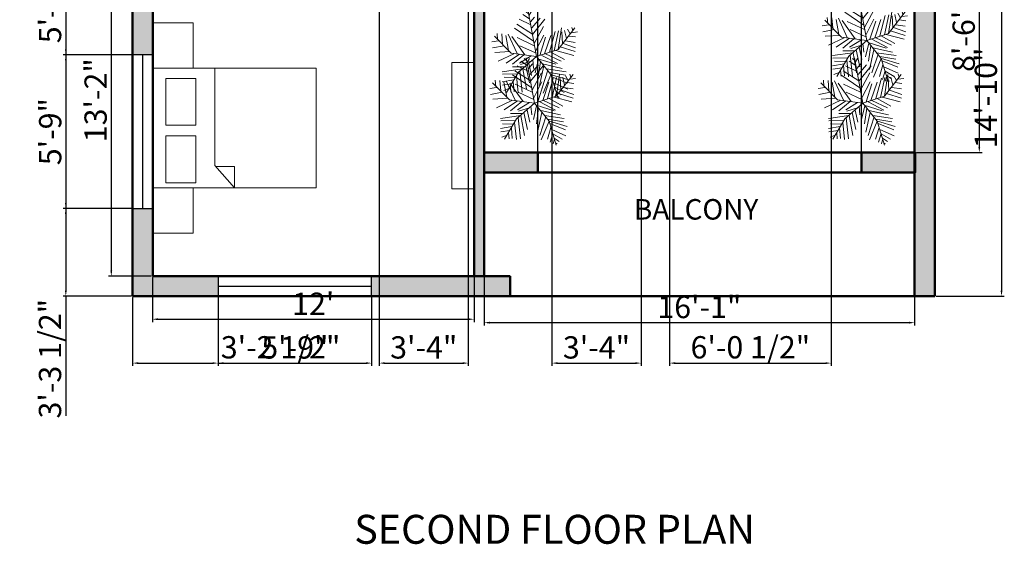
# Model space of a CAD drawing. Units: inches. Extents: x 1344 to 2521, y 3236 to 4924.
# Tile 4 of 14: x 1968 to 2410, y 3236 to 3472. Entities that reach past the tile are written whole.
import ezdxf

# ---------------------------------------------------------------- set-up
doc = ezdxf.new("R2010")
doc.units = ezdxf.units.IN
for name, color, linetype, lineweight in [('A-ANNO-DIMS', 2, 'Continuous', 18), ('A-ANNO-TEXT', 7, 'Continuous', 25), ('A-AREA-IDEN', 3, 'Continuous', 18), ('A-FURN', 130, 'Continuous', 18), ('A-GLAZ', 150, 'Continuous', 25), ('A-WALL', 31, 'Continuous', 50), ('A-WALL-PATT', 8, 'Continuous', 13), ('L-PLNT', 82, 'Continuous', 13)]:
    doc.layers.add(name, color=color, linetype=linetype, lineweight=lineweight)
doc.styles.get("Standard").update_dxf_attribs({"font": 'arial.ttf'})
doc.dimstyles.new('ISO-25', dxfattribs={"dimtxt": 10, "dimasz": 2.5, "dimexe": 1.25, "dimexo": 0.625, "dimtad": 1, "dimdec": 0, "dimlunit": 4, "dimtxsty": 'Standard', "dimcen": 2.5, "dimadec": 0, "dimazin": 0, "dimtfac": 1, "dimtdec": 0, "dimtmove": 0, "dimatfit": 3, "dimfxl": 1, "dimarcsym": 0})

# ---------------------------------------------------------------- blocks, each defined once
blk = doc.blocks.new('*U8')
for p, q in [((-8.737, 47.138), (-17.069, 52.711)), ((-10.186, 53.64), (-13.084, 55.962)), ((0, 0), (-10.5, 57)), ((-9.099, 51.782), (-6.563, 55.962)), ((-7.65, 43.423), (-2.578, 49.46)), ((-5.114, 28.097), (-24.676, 40.636)), ((-7.288, 39.707), (-21.778, 46.673)), ((-5.839, 35.992), (4.667, 48.067)), ((-5.114, 27.632), (10.463, 46.673)), ((-2.941, 16.486), (8.652, 37.85)), ((-31.5, 4.5), (-52.5, 25.5)), ((-48.585, 21.131), (-49.309, 29.026)), ((-43.513, 28.561), (-42.427, 15.558)), ((-38.442, 26.239), (-34.819, 7.663)), ((-35.544, 28.097), (-24.314, 3.947)), ((-14.533, 2.09), (-30.834, 25.31)), ((-3.665, 19.273), (-27.574, 35.527)), ((-1.129, 6.734), (9.014, 26.704)), ((10.101, 3.483), (17.708, 26.239)), ((16.259, 5.805), (23.142, 31.348)), ((22.055, 7.198), (27.489, 32.277)), ((27, 9), (48, 36)), ((27.127, 9.056), (31.112, 35.992)), ((31.836, 30.883), (32.561, 16.486)), ((35.096, 32.741), (37.27, 22.524)), ((38.719, 34.134), (41.979, 28.561)), ((40.53, 25.775), (48.862, 24.846)), ((43.791, 29.954), (51.036, 30.883)), ((44.153, 36.456), (45.239, 32.741)), ((-47.498, 19.737), (-55.83, 18.344)), ((-40.615, 13.7), (-55.105, 10.913)), ((-24.314, 23.917), (-2.941, 13.7)), ((-20.691, 13.7), (-1.129, 4.876)), ((3.942, 1.625), (11.187, 24.381)), ((29.662, 12.307), (48.137, 6.269)), ((33.285, 16.486), (48.862, 10.913)), ((36.183, 19.737), (48.137, 17.88)), ((-33.37, 6.269), (-52.207, 5.34)), ((-28.299, 3.483), (-47.86, -5.805)), ((-21.416, 3.018), (-38.079, -8.128)), ((0, 0), (-31.5, 4.5)), ((-15.982, 2.09), (-30.11, -9.521)), ((0, 0), (-22.5, -19.5)), ((-6.563, 1.161), (-21.416, -8.128)), ((0, 0), (27, 9)), ((0, 0), (18, -22.5)), ((6.478, 1.625), (26.04, -8.592)), ((11.187, 3.483), (30.749, -5.805)), ((18.07, 5.805), (35.096, -3.483)), ((24.229, 7.663), (46.688, 1.625)), ((-6.563, -5.805), (-19.967, -9.985)), ((-13.446, -11.378), (-8.737, -32.741)), ((-9.461, -8.592), (-6.201, -23.453)), ((-4.752, -3.483), (-3.665, -14.629)), ((2.493, -3.019), (-1.491, -20.202)), ((1.769, -2.555), (24.229, -9.521)), ((5.029, -6.27), (2.131, -25.775)), ((9.014, -11.378), (3.58, -35.992)), ((7.565, -9.056), (32.198, -14.629)), ((-17.431, -15.094), (-42.789, -18.809)), ((-24.314, -21.596), (-42.427, -22.06)), ((-22.5, -19.5), (-37.5, -45)), ((-15.257, -12.772), (-30.11, -12.772)), ((-25.038, -23.918), (-22.865, -45.281)), ((-20.691, -18.345), (-17.793, -44.352)), ((-17.069, -15.094), (-12.721, -40.172)), ((14.085, -16.951), (6.478, -40.172)), ((18.07, -22.524), (8.289, -45.745)), ((12.274, -15.094), (36.907, -18.809)), ((16.259, -19.738), (36.183, -22.989)), ((18, -22.5), (27, -52.5)), ((18.433, -22.524), (40.53, -29.026)), ((-28.299, -29.026), (-42.789, -31.348)), ((-30.834, -34.135), (-42.427, -35.528)), ((-26.849, -26.24), (-40.253, -25.775)), ((-29.023, -30.884), (-27.936, -43.887)), ((20.244, -30.419), (15.897, -44.816)), ((19.157, -25.311), (38.719, -33.206)), ((21.331, -32.741), (39.081, -40.636)), ((-34.457, -39.708), (-40.978, -42.494)), ((-32.646, -36.921), (-31.921, -44.352)), ((22.78, -37.85), (19.519, -48.532)), ((22.78, -38.314), (34.372, -44.816)), ((24.591, -45.745), (23.142, -50.854)), ((24.591, -43.423), (30.749, -47.603)), ((26.764, -49.925), (28.213, -50.854))]:
    blk.add_line(p, q)
blk = doc.blocks.new('*D54')
at = {"layer": 'A-ANNO-DIMS', "color": 0, "lineweight": -2, "transparency": 16777216}
for p, q in [((2026.74, 3514.45), (2007.52, 3514.45)), ((2008.77, 3511.95), (2008.77, 3358.97)), ((2026.74, 3356.47), (2007.52, 3356.47))]:
    blk.add_line(p, q, dxfattribs=at)
at = {"layer": 'A-ANNO-DIMS', "color": 0, "lineweight": 100, "transparency": 16777216}
for points in [[(2008.35, 3511.95), (2009.18, 3511.95), (2008.77, 3514.45)], [(2008.35, 3358.97), (2009.18, 3358.97), (2008.77, 3356.47)]]:
    blk.add_solid(points, dxfattribs=at)
at = {"layer": 'Defpoints', "color": 0, "lineweight": 100, "transparency": 16777216}
for p in [(2027.36, 3514.45), (2008.77, 3356.47), (2027.36, 3356.47)]:
    blk.add_point(p, dxfattribs=at)
at = {"layer": 'A-ANNO-DIMS', "color": 0, "transparency": 16777216, "insert": (2003.03, 3435.46), "char_height": 10, "attachment_point": 5, "rotation": 90}
blk.add_mtext('13\'-2"', dxfattribs=at)
blk = doc.blocks.new('*D55')
at = {"layer": 'A-ANNO-DIMS', "color": 0, "lineweight": -2, "transparency": 16777216}
for p, q in [((2027.24, 3355.85), (2027.24, 3335.92)), ((2171.6, 3355.85), (2171.6, 3335.92)), ((2029.74, 3337.17), (2169.1, 3337.17))]:
    blk.add_line(p, q, dxfattribs=at)
at = {"layer": 'A-ANNO-DIMS', "color": 0, "lineweight": 100, "transparency": 16777216}
for points in [[(2029.74, 3337.59), (2029.74, 3336.75), (2027.24, 3337.17)], [(2169.1, 3337.59), (2169.1, 3336.75), (2171.6, 3337.17)]]:
    blk.add_solid(points, dxfattribs=at)
at = {"layer": 'Defpoints', "color": 0, "lineweight": 100, "transparency": 16777216}
for p in [(2027.24, 3356.47), (2171.6, 3356.47), (2171.6, 3337.17)]:
    blk.add_point(p, dxfattribs=at)
at = {"layer": 'A-ANNO-DIMS', "color": 0, "transparency": 16777216, "insert": (2099.42, 3342.81), "char_height": 10, "attachment_point": 5}
blk.add_mtext("12'", dxfattribs=at)
blk = doc.blocks.new('*D56')
at = {"layer": 'A-ANNO-DIMS', "color": 0, "lineweight": -2, "transparency": 16777216}
for p, q in [((2176.1, 3355.85), (2176.1, 3334.38)), ((2369.36, 3355.89), (2369.36, 3334.38)), ((2178.6, 3335.63), (2366.86, 3335.63))]:
    blk.add_line(p, q, dxfattribs=at)
at = {"layer": 'A-ANNO-DIMS', "color": 0, "lineweight": 100, "transparency": 16777216}
for points in [[(2178.6, 3336.04), (2178.6, 3335.21), (2176.1, 3335.63)], [(2366.86, 3336.04), (2366.86, 3335.21), (2369.36, 3335.63)]]:
    blk.add_solid(points, dxfattribs=at)
at = {"layer": 'Defpoints', "color": 0, "lineweight": 100, "transparency": 16777216}
for p in [(2176.1, 3356.47), (2369.36, 3356.51), (2369.36, 3335.63)]:
    blk.add_point(p, dxfattribs=at)
at = {"layer": 'A-ANNO-DIMS', "color": 0, "transparency": 16777216, "insert": (2272.73, 3341.36), "char_height": 10, "attachment_point": 5}
blk.add_mtext('16\'-1"', dxfattribs=at)
blk = doc.blocks.new('*D59')
at = {"layer": 'A-ANNO-DIMS', "color": 0, "lineweight": -2, "transparency": 16777216}
for p, q in [((2369.99, 3514.45), (2399.65, 3514.45)), ((2398.4, 3511.95), (2398.4, 3414.51)), ((2370.19, 3412.01), (2399.65, 3412.01))]:
    blk.add_line(p, q, dxfattribs=at)
at = {"layer": 'A-ANNO-DIMS', "color": 0, "lineweight": 100, "transparency": 16777216}
for points in [[(2397.98, 3511.95), (2398.82, 3511.95), (2398.4, 3514.45)], [(2397.98, 3414.51), (2398.82, 3414.51), (2398.4, 3412.01)]]:
    blk.add_solid(points, dxfattribs=at)
at = {"layer": 'Defpoints', "color": 0, "lineweight": 100, "transparency": 16777216}
for p in [(2369.36, 3514.45), (2369.57, 3412.01), (2398.4, 3412.01)]:
    blk.add_point(p, dxfattribs=at)
at = {"layer": 'A-ANNO-DIMS', "color": 0, "transparency": 16777216, "insert": (2392.67, 3463.23), "char_height": 10, "attachment_point": 5, "rotation": 90}
blk.add_mtext('8\'-6"', dxfattribs=at)
blk = doc.blocks.new('BED-DOUBLE')
for p, q in [((27.95, 53.78), (27.95, 9.98)), ((27.95, 9.98), (36.68, 0)), ((36.68, 9.56), (28.32, 9.56)), ((36.68, 0), (36.68, 9.56))]:
    blk.add_line(p, q)
for points in [[(0, 0), (73.35, 0), (73.35, 53.78), (0, 53.78)], [(5.91, 28.08), (19.39, 28.08), (19.39, 49.13), (5.91, 49.13)], [(5.91, 2.27), (19.39, 2.27), (19.39, 23.31), (5.91, 23.31)]]:
    blk.add_lwpolyline(points, close=True)
blk = doc.blocks.new('*D186')
at = {"layer": 'A-ANNO-DIMS', "color": 0, "lineweight": -2, "transparency": 16777216}
for p, q in [((2017.74, 3763.43), (1987.11, 3763.43)), ((1988.36, 3760.93), (1988.36, 3350.01)), ((2017.74, 3347.51), (1987.11, 3347.51))]:
    blk.add_line(p, q, dxfattribs=at)
at = {"layer": 'A-ANNO-DIMS', "color": 0, "lineweight": 100, "transparency": 16777216}
for points in [[(1987.95, 3760.93), (1988.78, 3760.93), (1988.36, 3763.43)], [(1987.95, 3350.01), (1988.78, 3350.01), (1988.36, 3347.51)]]:
    blk.add_solid(points, dxfattribs=at)
at = {"layer": 'Defpoints', "color": 0, "lineweight": 100, "transparency": 16777216}
for p in [(2018.36, 3763.43), (1988.36, 3347.51), (2018.36, 3347.51)]:
    blk.add_point(p, dxfattribs=at)
at = {"layer": 'A-ANNO-DIMS', "color": 0, "transparency": 16777216, "insert": (1982.63, 3555.47), "char_height": 10, "attachment_point": 5, "rotation": 90}
blk.add_mtext('34\'-8"', dxfattribs=at)
blk = doc.blocks.new('*D200')
at = {"layer": 'A-ANNO-DIMS', "color": 0, "lineweight": -2, "transparency": 16777216}
for p, q in [((2017.74, 3527.47), (1987.11, 3527.47)), ((1988.36, 3524.97), (1988.36, 3458.32)), ((2017.74, 3455.82), (1987.11, 3455.82))]:
    blk.add_line(p, q, dxfattribs=at)
at = {"layer": 'A-ANNO-DIMS', "color": 0, "lineweight": 100, "transparency": 16777216}
for points in [[(1987.95, 3524.97), (1988.78, 3524.97), (1988.36, 3527.47)], [(1987.95, 3458.32), (1988.78, 3458.32), (1988.36, 3455.82)]]:
    blk.add_solid(points, dxfattribs=at)
at = {"layer": 'Defpoints', "color": 0, "lineweight": 100, "transparency": 16777216}
for p in [(2018.36, 3527.47), (1988.36, 3455.82), (2018.36, 3455.82)]:
    blk.add_point(p, dxfattribs=at)
at = {"layer": 'A-ANNO-DIMS', "color": 0, "transparency": 16777216, "insert": (1982.57, 3491.65), "char_height": 10, "attachment_point": 5, "rotation": 90}
blk.add_mtext('5\'-11 1/2"', dxfattribs=at)
blk = doc.blocks.new('*D201')
at = {"layer": 'A-ANNO-DIMS', "color": 0, "lineweight": -2, "transparency": 16777216}
for p, q in [((2017.74, 3455.82), (1987.11, 3455.82)), ((1988.36, 3453.32), (1988.36, 3389.4)), ((2017.74, 3386.9), (1987.11, 3386.9))]:
    blk.add_line(p, q, dxfattribs=at)
at = {"layer": 'A-ANNO-DIMS', "color": 0, "lineweight": 100, "transparency": 16777216}
for points in [[(1987.95, 3453.32), (1988.78, 3453.32), (1988.36, 3455.82)], [(1987.95, 3389.4), (1988.78, 3389.4), (1988.36, 3386.9)]]:
    blk.add_solid(points, dxfattribs=at)
at = {"layer": 'Defpoints', "color": 0, "lineweight": 100, "transparency": 16777216}
for p in [(2018.36, 3455.82), (1988.36, 3386.9), (2018.36, 3386.9)]:
    blk.add_point(p, dxfattribs=at)
at = {"layer": 'A-ANNO-DIMS', "color": 0, "transparency": 16777216, "insert": (1982.63, 3421.36), "char_height": 10, "attachment_point": 5, "rotation": 90}
blk.add_mtext('5\'-9"', dxfattribs=at)
blk = doc.blocks.new('*D202')
at = {"layer": 'A-ANNO-DIMS', "color": 0, "lineweight": -2, "transparency": 16777216}
for p, q in [((2017.74, 3386.9), (1987.11, 3386.9)), ((1988.36, 3384.4), (1988.36, 3350.01)), ((2017.74, 3347.51), (1987.11, 3347.51)), ((1988.36, 3347.51), (1988.36, 3293.88))]:
    blk.add_line(p, q, dxfattribs=at)
at = {"layer": 'A-ANNO-DIMS', "color": 0, "lineweight": 100, "transparency": 16777216}
for points in [[(1987.95, 3384.4), (1988.78, 3384.4), (1988.36, 3386.9)], [(1987.95, 3350.01), (1988.78, 3350.01), (1988.36, 3347.51)]]:
    blk.add_solid(points, dxfattribs=at)
at = {"layer": 'Defpoints', "color": 0, "lineweight": 100, "transparency": 16777216}
for p in [(2018.36, 3386.9), (1988.36, 3347.51), (2018.36, 3347.51)]:
    blk.add_point(p, dxfattribs=at)
at = {"layer": 'A-ANNO-DIMS', "color": 0, "transparency": 16777216, "insert": (1982.56, 3319.45), "char_height": 10, "attachment_point": 5, "rotation": 90}
blk.add_mtext('3\'-3 1/2"', dxfattribs=at)
blk = doc.blocks.new('*D205')
at = {"layer": 'A-ANNO-DIMS', "color": 0, "lineweight": -2, "transparency": 16777216}
for p, q in [((2378.99, 3525.36), (2409.61, 3525.36)), ((2408.36, 3522.86), (2408.36, 3350.01)), ((2378.99, 3347.51), (2409.61, 3347.51))]:
    blk.add_line(p, q, dxfattribs=at)
at = {"layer": 'A-ANNO-DIMS', "color": 0, "lineweight": 100, "transparency": 16777216}
for points in [[(2407.95, 3522.86), (2408.78, 3522.86), (2408.36, 3525.36)], [(2407.95, 3350.01), (2408.78, 3350.01), (2408.36, 3347.51)]]:
    blk.add_solid(points, dxfattribs=at)
at = {"layer": 'Defpoints', "color": 0, "lineweight": 100, "transparency": 16777216}
for p in [(2378.36, 3525.36), (2378.36, 3347.51), (2408.36, 3347.51)]:
    blk.add_point(p, dxfattribs=at)
at = {"layer": 'A-ANNO-DIMS', "color": 0, "transparency": 16777216, "insert": (2402.63, 3436.44), "char_height": 10, "attachment_point": 5, "rotation": 90}
blk.add_mtext('14\'-10"', dxfattribs=at)
blk = doc.blocks.new('*D206')
at = {"layer": 'A-ANNO-DIMS', "color": 0, "lineweight": -2, "transparency": 16777216}
for p, q in [((2018.36, 3346.89), (2018.36, 3316.22)), ((2056.7, 3346.85), (2056.7, 3316.22)), ((2020.86, 3317.47), (2054.2, 3317.47)), ((2056.7, 3317.47), (2110.32, 3317.47))]:
    blk.add_line(p, q, dxfattribs=at)
at = {"layer": 'A-ANNO-DIMS', "color": 0, "lineweight": 100, "transparency": 16777216}
for points in [[(2020.86, 3317.89), (2020.86, 3317.06), (2018.36, 3317.47)], [(2054.2, 3317.89), (2054.2, 3317.06), (2056.7, 3317.47)]]:
    blk.add_solid(points, dxfattribs=at)
at = {"layer": 'Defpoints', "color": 0, "lineweight": 100, "transparency": 16777216}
for p in [(2018.36, 3347.51), (2056.7, 3347.47), (2056.7, 3317.47)]:
    blk.add_point(p, dxfattribs=at)
at = {"layer": 'A-ANNO-DIMS', "color": 0, "transparency": 16777216, "insert": (2084.76, 3323.27), "char_height": 10, "attachment_point": 5}
blk.add_mtext('3\'-2 1/2"', dxfattribs=at)
blk = doc.blocks.new('*D207')
at = {"layer": 'A-ANNO-DIMS', "color": 0, "lineweight": -2, "transparency": 16777216}
for p, q in [((2056.7, 3346.85), (2056.7, 3316.22)), ((2125.62, 3346.85), (2125.62, 3316.22)), ((2059.2, 3317.47), (2123.12, 3317.47))]:
    blk.add_line(p, q, dxfattribs=at)
at = {"layer": 'A-ANNO-DIMS', "color": 0, "lineweight": 100, "transparency": 16777216}
for points in [[(2059.2, 3317.89), (2059.2, 3317.06), (2056.7, 3317.47)], [(2123.12, 3317.89), (2123.12, 3317.06), (2125.62, 3317.47)]]:
    blk.add_solid(points, dxfattribs=at)
at = {"layer": 'Defpoints', "color": 0, "lineweight": 100, "transparency": 16777216}
for p in [(2056.7, 3347.47), (2125.62, 3347.47), (2125.62, 3317.47)]:
    blk.add_point(p, dxfattribs=at)
at = {"layer": 'A-ANNO-DIMS', "color": 0, "transparency": 16777216, "insert": (2091.16, 3323.2), "char_height": 10, "attachment_point": 5}
blk.add_mtext('5\'-9"', dxfattribs=at)
blk = doc.blocks.new('*D209')
at = {"layer": 'A-ANNO-DIMS', "color": 0, "lineweight": -2, "transparency": 16777216}
for p, q in [((2129.02, 3619.06), (2129.02, 3316.22)), ((2169.02, 3619.06), (2169.02, 3316.22)), ((2131.52, 3317.47), (2166.52, 3317.47))]:
    blk.add_line(p, q, dxfattribs=at)
at = {"layer": 'A-ANNO-DIMS', "color": 0, "lineweight": 100, "transparency": 16777216}
for points in [[(2131.52, 3317.89), (2131.52, 3317.06), (2129.02, 3317.47)], [(2166.52, 3317.89), (2166.52, 3317.06), (2169.02, 3317.47)]]:
    blk.add_solid(points, dxfattribs=at)
at = {"layer": 'Defpoints', "color": 0, "lineweight": 100, "transparency": 16777216}
for p in [(2129.02, 3619.69), (2169.02, 3619.69), (2169.02, 3317.47)]:
    blk.add_point(p, dxfattribs=at)
at = {"layer": 'A-ANNO-DIMS', "color": 0, "transparency": 16777216, "insert": (2149.02, 3323.21), "char_height": 10, "attachment_point": 5}
blk.add_mtext('3\'-4"', dxfattribs=at)
blk = doc.blocks.new('*D215')
at = {"layer": 'A-ANNO-DIMS', "color": 0, "lineweight": -2, "transparency": 16777216}
for p, q in [((2206.56, 3513.82), (2206.56, 3316.22)), ((2246.56, 3513.82), (2246.56, 3316.22)), ((2209.06, 3317.47), (2244.06, 3317.47))]:
    blk.add_line(p, q, dxfattribs=at)
at = {"layer": 'A-ANNO-DIMS', "color": 0, "lineweight": 100, "transparency": 16777216}
for points in [[(2209.06, 3317.89), (2209.06, 3317.06), (2206.56, 3317.47)], [(2244.06, 3317.89), (2244.06, 3317.06), (2246.56, 3317.47)]]:
    blk.add_solid(points, dxfattribs=at)
at = {"layer": 'Defpoints', "color": 0, "lineweight": 100, "transparency": 16777216}
for p in [(2206.56, 3514.45), (2246.56, 3514.45), (2246.56, 3317.47)]:
    blk.add_point(p, dxfattribs=at)
at = {"layer": 'A-ANNO-DIMS', "color": 0, "transparency": 16777216, "insert": (2226.56, 3323.21), "char_height": 10, "attachment_point": 5}
blk.add_mtext('3\'-4"', dxfattribs=at)
blk = doc.blocks.new('*D216')
at = {"layer": 'A-ANNO-DIMS', "color": 0, "lineweight": -2, "transparency": 16777216}
for p, q in [((2176.1, 3403.64), (2176.1, 3794.68)), ((2178.6, 3793.43), (2197.7, 3793.43)), ((2200.2, 3403.64), (2200.2, 3794.68)), ((2200.2, 3793.43), (2230.7, 3793.43))]:
    blk.add_line(p, q, dxfattribs=at)
at = {"layer": 'A-ANNO-DIMS', "color": 0, "lineweight": 100, "transparency": 16777216}
for points in [[(2178.6, 3793.85), (2178.6, 3793.02), (2176.1, 3793.43)], [(2197.7, 3793.85), (2197.7, 3793.02), (2200.2, 3793.43)]]:
    blk.add_solid(points, dxfattribs=at)
at = {"layer": 'Defpoints', "color": 0, "lineweight": 100, "transparency": 16777216}
for p in [(2200.2, 3793.43), (2176.1, 3403.01), (2200.2, 3403.01)]:
    blk.add_point(p, dxfattribs=at)
at = {"layer": 'A-ANNO-DIMS', "color": 0, "transparency": 16777216, "insert": (2216.7, 3799.16), "char_height": 10, "attachment_point": 5}
blk.add_mtext('2\'-0"', dxfattribs=at)
blk = doc.blocks.new('*D217')
at = {"layer": 'A-ANNO-DIMS', "color": 0, "lineweight": -2, "transparency": 16777216}
for p, q in [((2200.2, 3403.64), (2200.2, 3794.68)), ((2202.7, 3793.43), (2342.96, 3793.43)), ((2345.46, 3403.64), (2345.46, 3794.68))]:
    blk.add_line(p, q, dxfattribs=at)
at = {"layer": 'A-ANNO-DIMS', "color": 0, "lineweight": 100, "transparency": 16777216}
for points in [[(2202.7, 3793.85), (2202.7, 3793.02), (2200.2, 3793.43)], [(2342.96, 3793.85), (2342.96, 3793.02), (2345.46, 3793.43)]]:
    blk.add_solid(points, dxfattribs=at)
at = {"layer": 'Defpoints', "color": 0, "lineweight": 100, "transparency": 16777216}
for p in [(2345.46, 3793.43), (2200.2, 3403.01), (2345.46, 3403.01)]:
    blk.add_point(p, dxfattribs=at)
at = {"layer": 'A-ANNO-DIMS', "color": 0, "transparency": 16777216, "insert": (2272.83, 3799.23), "char_height": 10, "attachment_point": 5}
blk.add_mtext('12\'-1 1/2"', dxfattribs=at)
blk = doc.blocks.new('*D218')
at = {"layer": 'A-ANNO-DIMS', "color": 0, "lineweight": -2, "transparency": 16777216}
for p, q in [((2259.38, 3518.32), (2259.38, 3316.22)), ((2331.86, 3518.32), (2331.86, 3316.22)), ((2261.88, 3317.47), (2329.36, 3317.47))]:
    blk.add_line(p, q, dxfattribs=at)
at = {"layer": 'A-ANNO-DIMS', "color": 0, "lineweight": 100, "transparency": 16777216}
for points in [[(2261.88, 3317.89), (2261.88, 3317.06), (2259.38, 3317.47)], [(2329.36, 3317.89), (2329.36, 3317.06), (2331.86, 3317.47)]]:
    blk.add_solid(points, dxfattribs=at)
at = {"layer": 'Defpoints', "color": 0, "lineweight": 100, "transparency": 16777216}
for p in [(2259.38, 3518.95), (2331.86, 3518.95), (2331.86, 3317.47)]:
    blk.add_point(p, dxfattribs=at)
at = {"layer": 'A-ANNO-DIMS', "color": 0, "transparency": 16777216, "insert": (2295.62, 3323.27), "char_height": 10, "attachment_point": 5}
blk.add_mtext('6\'-0 1/2"', dxfattribs=at)

msp = doc.modelspace()

# ---------------------------------------------------------------- hatches: boundary and pattern name
at = {"layer": 'A-WALL-PATT'}
h = msp.add_hatch(color=256, dxfattribs=at)
h.dxf.hatch_style = 1
h.paths.add_polyline_path([(2193.45, 3763.43), (2126.57, 3763.43), (2126.57, 3754.43), (2193.45, 3754.43)])
h.paths.add_polyline_path([(2057.65, 3763.43), (2018.36, 3763.43), (2018.36, 3608.87), (2027.36, 3608.87), (2027.36, 3754.43), (2057.65, 3754.43)])
h.paths.add_polyline_path([(2266.48, 3763.43), (2226.56, 3763.43), (2226.56, 3754.43), (2266.48, 3754.43)])
h.paths.add_polyline_path([(2378.36, 3763.43), (2335.41, 3763.43), (2335.41, 3754.43), (2369.36, 3754.43), (2369.36, 3594.28), (2378.36, 3594.28)])
h.paths.add_polyline_path([(2369.36, 3610.02), (2250.29, 3610.02), (2250.29, 3605.52), (2369.36, 3605.52)])
h.paths.add_polyline_path([(2250.29, 3610.02), (2245.79, 3610.02), (2245.79, 3605.52), (2250.29, 3605.52)])
h.paths.add_polyline_path([(2250.29, 3754.43), (2245.79, 3754.43), (2245.79, 3655.04), (2250.29, 3655.04)])
h.paths.add_polyline_path([(2176.1, 3754.43), (2171.6, 3754.43), (2171.6, 3624.19), (2171.35, 3624.19), (2169.02, 3624.19), (2169.02, 3619.69), (2176.1, 3619.69)])
h.paths.add_polyline_path([(2129.02, 3624.19), (2122.52, 3624.19), (2122.52, 3619.69), (2129.02, 3619.69)])
h.paths.add_polyline_path([(2091.69, 3624.19), (2027.36, 3624.19), (2027.36, 3619.69), (2091.72, 3619.69, -0.012876), (2091.69, 3620.84)])
h.paths.add_polyline_path([(2250.29, 3615.04), (2245.79, 3615.04), (2245.79, 3610.02), (2250.29, 3610.02)])
h.paths.add_polyline_path([(2027.36, 3580.89), (2018.36, 3580.89), (2018.36, 3555.45), (2027.36, 3555.45)])
h.paths.add_polyline_path([(2027.36, 3527.47), (2018.36, 3527.47), (2018.36, 3455.82), (2027.36, 3455.82)])
h.paths.add_polyline_path([(2093.06, 3517.8, -0.012876), (2093.09, 3518.95), (2027.36, 3518.95), (2027.36, 3514.45), (2093.06, 3514.45)])
h.paths.add_polyline_path([(2118.02, 3573.32), (2110.02, 3573.32), (2110.02, 3573.28), (2080.51, 3573.28), (2027.36, 3573.32), (2027.36, 3568.82), (2118.02, 3568.82)])
h.paths.add_polyline_path([(2122.52, 3624.19), (2114.02, 3624.19), (2114.02, 3620.84), (2114.02, 3619.69), (2118.02, 3619.69), (2118.02, 3518.95), (2122.52, 3518.95)])
h.paths.add_polyline_path([(2129.02, 3518.95), (2115.39, 3518.95), (2115.39, 3517.8), (2115.39, 3514.45), (2129.02, 3514.45)])
h.paths.add_polyline_path([(2027.36, 3386.9), (2018.36, 3386.9), (2018.36, 3347.51), (2056.7, 3347.51), (2056.7, 3356.47), (2027.36, 3356.47)])
h.paths.add_polyline_path([(2187.76, 3356.47), (2168.81, 3356.47), (2149.67, 3356.47), (2125.62, 3356.47), (2125.62, 3347.51), (2176.1, 3347.51), (2187.76, 3347.51)])
h.paths.add_polyline_path([(2378.36, 3525.36), (2369.36, 3525.36), (2369.36, 3497.27), (2369.36, 3412.01), (2369.57, 3412.01), (2369.57, 3403.01), (2369.36, 3356.51), (2369.36, 3347.51), (2378.36, 3347.51)])
h.paths.add_polyline_path([(2369.36, 3412.01), (2345.46, 3412.01), (2345.46, 3403.01), (2369.36, 3403.01)])
h.paths.add_polyline_path([(2206.56, 3518.95), (2176.1, 3518.95), (2176.1, 3514.45), (2206.56, 3514.45)])
h.paths.add_polyline_path([(2130.92, 3560.64), (2239.92, 3560.64), (2239.92, 3579.62), (2130.92, 3579.62)], flags=9)
h.paths.add_polyline_path([(2271.24, 3730.09), (2345.91, 3730.09), (2345.91, 3749.07), (2271.24, 3749.07)], flags=9)
h.paths.add_polyline_path([(2051.28, 3467.76), (2122.39, 3467.76), (2122.39, 3502.26), (2051.28, 3502.26)], flags=9)
h.paths.add_polyline_path([(2033.92, 3520.24), (2083.56, 3520.24), (2083.56, 3539.22), (2033.92, 3539.22)], flags=9)
h.paths.add_polyline_path([(2030.69, 3603.57), (2080.34, 3603.57), (2080.34, 3622.55), (2030.69, 3622.55)], flags=9)
h.paths.add_polyline_path([(2175.78, 3699.42), (2225.43, 3699.42), (2225.43, 3718.41), (2175.78, 3718.41)], flags=9)
h.paths.add_polyline_path([(2051.88, 3718.72), (2122.99, 3718.72), (2122.99, 3753.22), (2051.88, 3753.22)], flags=9)
h = msp.add_hatch(color=256, dxfattribs=at)
h.dxf.hatch_style = 1
h.paths.add_polyline_path([(2200.2, 3412.01), (2176.1, 3412.01), (2176.1, 3403.01), (2200.2, 3403.01)])
h.paths.add_polyline_path([(2369.36, 3518.95), (2246.56, 3518.95), (2246.56, 3514.45), (2369.36, 3514.45)])
h.paths.add_polyline_path([(2130.92, 3560.64), (2239.92, 3560.64), (2239.92, 3579.62), (2130.92, 3579.62)], flags=9)
h.paths.add_polyline_path([(2271.24, 3730.09), (2345.91, 3730.09), (2345.91, 3749.07), (2271.24, 3749.07)], flags=9)
h.paths.add_polyline_path([(2051.28, 3467.76), (2122.39, 3467.76), (2122.39, 3502.26), (2051.28, 3502.26)], flags=9)
h.paths.add_polyline_path([(2033.92, 3520.24), (2083.56, 3520.24), (2083.56, 3539.22), (2033.92, 3539.22)], flags=9)
h.paths.add_polyline_path([(2030.69, 3603.57), (2080.34, 3603.57), (2080.34, 3622.55), (2030.69, 3622.55)], flags=9)
h.paths.add_polyline_path([(2175.78, 3699.42), (2225.43, 3699.42), (2225.43, 3718.41), (2175.78, 3718.41)], flags=9)
h.paths.add_polyline_path([(2051.88, 3718.72), (2122.99, 3718.72), (2122.99, 3753.22), (2051.88, 3753.22)], flags=9)
h = msp.add_hatch(color=256, dxfattribs=at)
h.dxf.hatch_style = 1
h.paths.add_polyline_path([(2176.1, 3518.95), (2171.6, 3518.95), (2171.6, 3514.45), (2171.6, 3356.47), (2176.1, 3356.47)])
h.paths.add_polyline_path([(2171.6, 3518.95), (2169.02, 3518.95), (2169.02, 3514.45), (2171.6, 3514.45)])

# ---------------------------------------------------------------- linework, layer by layer
at = {"layer": 'A-FURN'}
for points in [[(2027.36, 3449.9), (2045.59, 3449.9), (2045.59, 3470.24), (2027.36, 3470.24)], [(2171.6, 3452.39), (2161.64, 3452.39), (2161.64, 3395.65), (2171.6, 3395.65)], [(2027.36, 3375.77), (2045.59, 3375.77), (2045.59, 3396.12), (2027.36, 3396.12)]]:
    msp.add_lwpolyline(points, close=True, dxfattribs=at)
at = {"layer": 'A-GLAZ'}
for p, q in [((2022.86, 3386.9), (2022.86, 3455.82)), ((2056.7, 3351.97), (2125.62, 3351.97))]:
    msp.add_line(p, q, dxfattribs=at)
for points in [[(2018.36, 3386.9), (2027.36, 3386.9), (2027.36, 3455.82), (2018.36, 3455.82)], [(2056.7, 3356.47), (2056.7, 3347.47), (2125.62, 3347.47), (2125.62, 3356.47)]]:
    msp.add_lwpolyline(points, close=True, dxfattribs=at)
at = {"layer": 'A-WALL'}
for p, q in [((2171.6, 3514.45), (2171.6, 3356.47)), ((2176.1, 3514.45), (2176.1, 3356.47)), ((2369.36, 3397.36), (2369.36, 3433.36)), ((2369.36, 3412.01), (2176.1, 3412.01)), ((2369.36, 3403.01), (2176.1, 3403.01)), ((2027.24, 3356.47), (2149.67, 3356.47)), ((2149.67, 3356.47), (2171.6, 3356.47)), ((2187.76, 3356.47), (2168.81, 3356.47)), ((2187.76, 3347.51), (2187.76, 3356.47)), ((2369.36, 3356.51), (2369.36, 3347.51)), ((2027.36, 3347.51), (2018.36, 3347.51)), ((2018.36, 3347.51), (2176.1, 3347.51)), ((2027.36, 3347.51), (2149.79, 3347.51)), ((2176.1, 3347.51), (2187.76, 3347.51)), ((2187.76, 3347.51), (2369.36, 3347.51)), ((2378.36, 3347.51), (2369.36, 3347.51)), ((2369.36, 3347.51), (2378.36, 3347.51))]:
    msp.add_line(p, q, dxfattribs=at)
for points in [[(2378.36, 3347.51), (2378.36, 3763.43), (2018.36, 3763.43), (2018.36, 3347.51)], [(2369.36, 3356.51), (2369.36, 3754.43), (2027.36, 3754.43), (2027.36, 3356.47)], [(2249.37, 3412.01), (2273.47, 3412.01)], [(2273.47, 3403.01), (2249.37, 3403.01)]]:
    msp.add_lwpolyline(points, dxfattribs=at)
for points in [[(2171.6, 3356.47), (2176.1, 3356.47), (2176.1, 3518.95), (2171.6, 3518.95)], [(2176.1, 3412.01), (2200.2, 3412.01), (2200.2, 3403.01), (2176.1, 3403.01)], [(2345.46, 3412.01), (2369.57, 3412.01), (2369.57, 3403.01), (2345.46, 3403.01)]]:
    msp.add_lwpolyline(points, close=True, dxfattribs=at)

# ---------------------------------------------------------------- block references
at = {"layer": 'A-FURN'}
msp.add_blockref('BED-DOUBLE', (2027.36, 3396.12), dxfattribs=at)
at = {"layer": 'L-PLNT', "xscale": 0.3591539065448135, "yscale": 0.3591539065448135, "zscale": 0.3591539065448135}
for p in [(2347.88, 3462.21), (2199.64, 3455.01), (2198.79, 3434.08), (2346.12, 3434.08)]:
    msp.add_blockref('*U8', p, dxfattribs=at)

# ---------------------------------------------------------------- texts
at = {"layer": 'A-ANNO-TEXT', "insert": (2117.83, 3249.38), "char_height": 12.9935, "attachment_point": 1}
msp.add_mtext_dynamic_manual_height_columns('SECOND FLOOR PLAN', width=2122.9296, gutter_width=64.97, heights=[0], dxfattribs=at)
at = {"layer": 'A-AREA-IDEN', "insert": (2243.37, 3391.09), "char_height": 9.211, "attachment_point": 1}
msp.add_mtext_dynamic_manual_height_columns('BALCONY', width=108.7809, gutter_width=46.06, heights=[0], dxfattribs=at)

# ---------------------------------------------------------------- dimensions: what is measured, and where the dimension line sits
at = {"layer": 'A-ANNO-DIMS'}
for base, p1, p2, override, picture, middle in [((2345.46, 3793.43), (2200.2, 3403.01), (2345.46, 3403.01), {"dimdec": 1, "dimlfac": 1, "dimrnd": 0, "dimzin": 1, "dimdsep": 46, "dimlunit": 4, "dimfrac": 2}, '*D217', (2272.83, 3799.23)), ((2200.2, 3793.43), (2176.1, 3403.01), (2200.2, 3403.01), {"dimdec": 1, "dimlfac": 1, "dimrnd": 0, "dimzin": 1, "dimdsep": 46, "dimlunit": 4, "dimfrac": 2}, '*D216', (2216.7, 3799.16)), ((2169.02, 3317.47), (2129.02, 3619.69), (2169.02, 3619.69), {"dimdec": 1, "dimlfac": 1, "dimrnd": 0, "dimzin": 1, "dimdsep": 46, "dimlunit": 4, "dimfrac": 2}, '*D209', (2149.02, 3323.21)), ((2331.86, 3317.47), (2259.38, 3518.95), (2331.86, 3518.95), {"dimdec": 1, "dimlfac": 1, "dimrnd": 0, "dimzin": 1, "dimdsep": 46, "dimlunit": 4, "dimfrac": 2}, '*D218', (2295.62, 3323.27)), ((2246.56, 3317.47), (2206.56, 3514.45), (2246.56, 3514.45), {"dimdec": 1, "dimlfac": 1, "dimrnd": 0, "dimzin": 1, "dimdsep": 46, "dimlunit": 4, "dimfrac": 2}, '*D215', (2226.56, 3323.21)), ((2171.6, 3337.17), (2027.24, 3356.47), (2171.6, 3356.47), {"dimclrd": 0, "dimclre": 0, "dimclrt": 0}, '*D55', (2099.42, 3342.81)), ((2369.36, 3335.63), (2176.1, 3356.47), (2369.36, 3356.51), {"dimclrd": 0, "dimclre": 0, "dimclrt": 0}, '*D56', (2272.73, 3341.36)), ((2056.7, 3317.47), (2018.36, 3347.51), (2056.7, 3347.47), {"dimdec": 1, "dimlfac": 1, "dimrnd": 0, "dimzin": 1, "dimdsep": 46, "dimlunit": 4, "dimfrac": 2}, '*D206', (2084.76, 3323.27)), ((2125.62, 3317.47), (2056.7, 3347.47), (2125.62, 3347.47), {"dimdec": 1, "dimlfac": 1, "dimrnd": 0, "dimzin": 1, "dimdsep": 46, "dimlunit": 4, "dimfrac": 2}, '*D207', (2091.16, 3323.2))]:
    dim = msp.add_linear_dim(base=base, p1=p1, p2=p2, dimstyle='ISO-25', override=override, dxfattribs=at)
    dim.commit()
    dim.dimension.update_dxf_attribs({"geometry": picture, "text_midpoint": middle})
for base, p1, p2, override, picture, middle in [((1988.36, 3347.51), (2018.36, 3763.43), (2018.36, 3347.51), {"dimdec": 1, "dimlfac": 1, "dimrnd": 0, "dimzin": 1, "dimdsep": 46, "dimlunit": 4, "dimfrac": 2}, '*D186', (1982.63, 3555.47)), ((1988.3631, 3455.8226), (2018.3631, 3527.4742), (2018.3631, 3455.8226), {"dimdec": 1, "dimlfac": 1, "dimrnd": 0, "dimzin": 1, "dimdsep": 46, "dimlunit": 4, "dimfrac": 2}, '*D200', (1982.5676, 3491.6484)), ((2408.3631, 3347.5114), (2378.3631, 3525.3602), (2378.3631, 3347.5114), {"dimdec": 1, "dimlfac": 1, "dimrnd": 0, "dimzin": 1, "dimdsep": 46, "dimlunit": 4, "dimfrac": 2}, '*D205', (2402.6324, 3436.4358)), ((2008.77, 3356.47), (2027.36, 3514.45), (2027.36, 3356.47), {"dimclrd": 0, "dimclre": 0, "dimclrt": 0}, '*D54', (2003.03, 3435.46)), ((2398.4, 3412.01), (2369.36, 3514.45), (2369.57, 3412.01), {"dimclrd": 0, "dimclre": 0, "dimclrt": 0}, '*D59', (2392.67, 3463.23)), ((1988.36, 3386.9), (2018.36, 3455.82), (2018.36, 3386.9), {"dimdec": 1, "dimlfac": 1, "dimrnd": 0, "dimzin": 1, "dimdsep": 46, "dimlunit": 4, "dimfrac": 2}, '*D201', (1982.63, 3421.36)), ((1988.36, 3347.51), (2018.36, 3386.9), (2018.36, 3347.51), {"dimdec": 1, "dimlfac": 1, "dimrnd": 0, "dimzin": 1, "dimdsep": 46, "dimlunit": 4, "dimfrac": 2}, '*D202', (1982.56, 3319.45))]:
    dim = msp.add_linear_dim(base=base, p1=p1, p2=p2, angle=90, dimstyle='ISO-25', override=override, dxfattribs=at)
    dim.commit()
    dim.dimension.update_dxf_attribs({"geometry": picture, "text_midpoint": middle})

doc.saveas('drawing.dxf')
